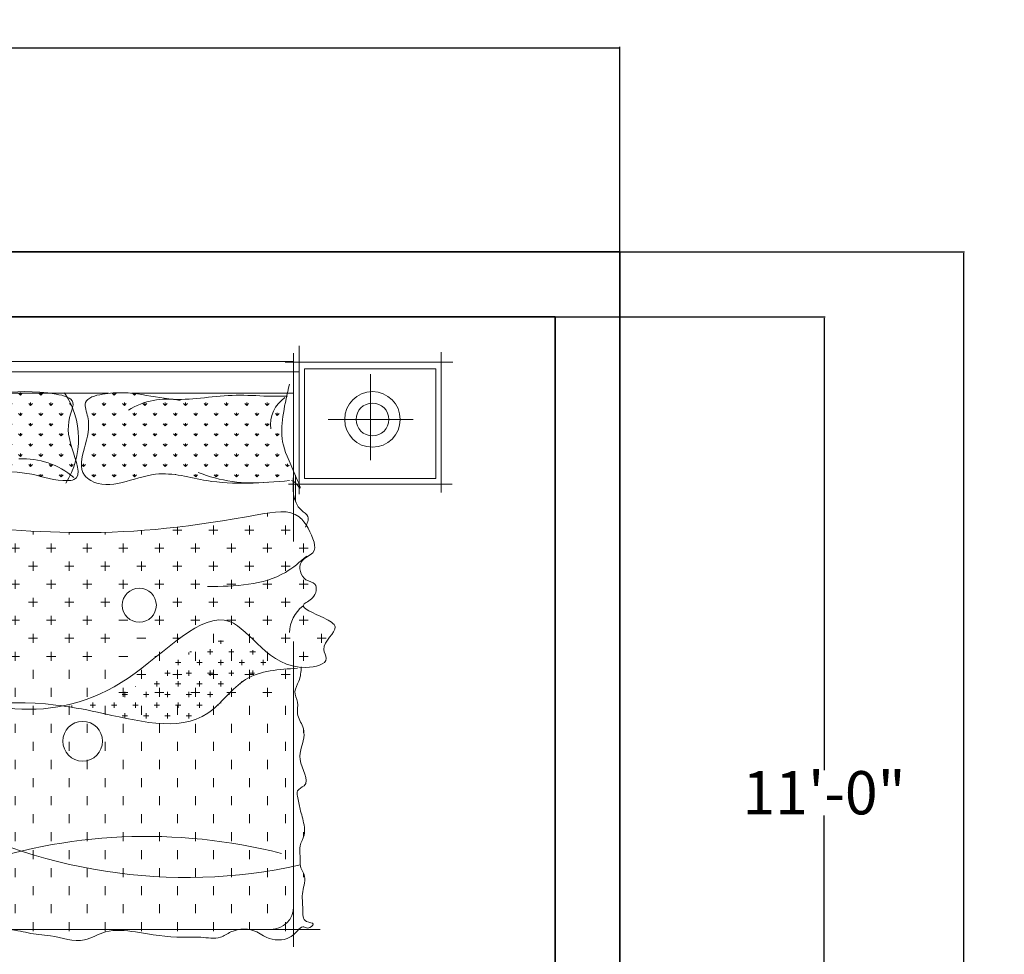
# Model space of a CAD drawing. Units: inches. Extents: x -26 to 575, y -18 to 513.
# Tile 28 of 28: x 439 to 575, y 378 to 508. Entities that reach past the tile are written whole.
import ezdxf

# ---------------------------------------------------------------- set-up
doc = ezdxf.new("R2010")
doc.units = ezdxf.units.IN
doc.header["$MEASUREMENT"] = 0
for name, color, linetype, lineweight in [('A-ANNO-DIMS', 2, 'Continuous', 18), ('A-WALL', 7, 'Continuous', 35), ('Furniture', 8, 'Continuous', 15)]:
    doc.layers.add(name, color=color, linetype=linetype, lineweight=lineweight)
doc.styles.get("Standard").update_dxf_attribs({"font": 'arial.ttf', "height": 6})
doc.dimstyles.get("Standard").update_dxf_attribs({"dimtxt": 6, "dimasz": 0.18, "dimexe": 0.18, "dimexo": 0.0625, "dimgap": 0.09, "dimtad": 0, "dimtih": 1, "dimtoh": 1, "dimzin": 0, "dimdsep": 46, "dimlunit": 3, "dimtxsty": 'Standard', "dimcen": 0.09, "dimadec": 0, "dimazin": 0, "dimtfac": 1, "dimtofl": 0, "dimtmove": 0, "dimatfit": 3, "dimfxl": 1, "dimtolj": 1, "dimtzin": 0, "dimarcsym": 0})

# ---------------------------------------------------------------- blocks, each defined once
blk = doc.blocks.new('*D1')
at = {"layer": 'A-ANNO-DIMS', "color": 0, "lineweight": -2, "transparency": 16777216}
for p, q in [((18.18, 475.57), (18.18, 503.94)), ((522.18, 475.57), (522.18, 503.94)), ((18.36, 503.76), (264.87, 503.76)), ((522, 503.76), (275.48, 503.76))]:
    blk.add_line(p, q, dxfattribs=at)
at = {"layer": 'A-ANNO-DIMS', "color": 0, "transparency": 16777216}
for points in [[(18.36, 503.79), (18.36, 503.73), (18.18, 503.76)], [(522, 503.79), (522, 503.73), (522.18, 503.76)]]:
    blk.add_solid(points, dxfattribs=at)
at = {"layer": 'Defpoints', "color": 0, "transparency": 16777216}
for p in [(522.18, 503.76), (18.18, 475.51), (522.18, 475.51)]:
    blk.add_point(p, dxfattribs=at)
at = {"layer": 'A-ANNO-DIMS', "color": 0, "transparency": 16777216, "insert": (270.18, 503.76), "char_height": 6, "attachment_point": 5}
blk.add_mtext("\\A1;42'", dxfattribs=at)
blk = doc.blocks.new('*D2')
at = {"layer": 'A-ANNO-DIMS', "color": 0, "lineweight": -2, "transparency": 16777216}
for p, q in [((522.24, 475.51), (569.98, 475.51)), ((569.8, 475.33), (569.8, 250.66)), ((569.8, 19.69), (569.8, 244.35)), ((522.24, 19.51), (569.98, 19.51))]:
    blk.add_line(p, q, dxfattribs=at)
at = {"layer": 'A-ANNO-DIMS', "color": 0, "transparency": 16777216}
for points in [[(569.77, 475.33), (569.83, 475.33), (569.8, 475.51)], [(569.77, 19.69), (569.83, 19.69), (569.8, 19.51)]]:
    blk.add_solid(points, dxfattribs=at)
at = {"layer": 'Defpoints', "color": 0, "transparency": 16777216}
for p in [(522.18, 475.51), (522.18, 19.51), (569.8, 19.51)]:
    blk.add_point(p, dxfattribs=at)
at = {"layer": 'A-ANNO-DIMS', "color": 0, "transparency": 16777216, "insert": (569.8, 247.51), "char_height": 6, "attachment_point": 5}
blk.add_mtext("\\A1;38'", dxfattribs=at)
blk = doc.blocks.new('BED-DOUBLE-WITH-NIGHTSTANDS')
for p, q in [((1.93, 83.36), (1.93, 62.76)), ((82.67, 83.36), (82.67, 62.76)), ((21.61, 63.03), (21.61, 82.46)), ((22.83, 60.83), (22.83, 82.62)), ((81.88, 82.34), (81.88, 56.23)), ((102.35, 63.03), (102.35, 82.46)), ((23.23, 81.08), (0, 81.08)), ((10.27, 81.76), (8.94, 70.83)), ((21.24, 81.17), (81.88, 81.17)), ((103.97, 81.08), (80.74, 81.08)), ((20.89, 80.15), (2.67, 80.15)), ((2.67, 80.15), (2.67, 64.97)), ((20.89, 64.97), (20.89, 80.15)), ((82.67, 79.72), (21.06, 79.72)), ((101.63, 80.15), (83.41, 80.15)), ((83.41, 80.15), (83.41, 64.97)), ((92.57, 79.4), (92.57, 67.51)), ((101.63, 64.97), (101.63, 80.15)), ((14.67, 76.01), (4.51, 77.26)), ((25.06, 76.76), (22.83, 76.76)), ((41.17, 76.51), (40.96, 76.72)), ((41.17, 76.51), (41.43, 76.77)), ((41.17, 76.51), (41.17, 76.74)), ((56.23, 76.76), (41.36, 76.76)), ((44, 76.51), (43.73, 76.77)), ((44, 76.51), (44, 76.88)), ((44, 76.51), (44.26, 76.77)), ((46.83, 76.51), (46.56, 76.77)), ((46.83, 76.51), (46.83, 76.88)), ((46.83, 76.51), (47.09, 76.77)), ((57, 76.51), (56.74, 76.77)), ((57, 76.51), (57, 76.83)), ((57, 76.51), (57.27, 76.77)), ((81.88, 76.76), (59.39, 76.76)), ((59.83, 76.51), (59.59, 76.74)), ((59.83, 76.51), (59.83, 76.72)), ((59.83, 76.51), (60.02, 76.69)), ((8.06, 67.24), (12.03, 75.72)), ((11.46, 75.32), (8.12, 68.2)), ((11.77, 75.18), (11.46, 75.32)), ((12.03, 75.72), (14.23, 74.69)), ((25.61, 75.09), (25.35, 75.36)), ((25.61, 75.09), (25.61, 75.47)), ((25.61, 75.09), (25.88, 75.36)), ((28.44, 75.09), (28.18, 75.36)), ((28.44, 75.09), (28.44, 75.47)), ((28.44, 75.09), (28.71, 75.36)), ((31.27, 75.09), (31, 75.36)), ((31.27, 75.09), (31.27, 75.47)), ((31.27, 75.09), (31.53, 75.36)), ((34.1, 75.09), (33.83, 75.36)), ((34.1, 75.09), (34.1, 75.47)), ((34.1, 75.09), (34.36, 75.36)), ((36.93, 75.09), (36.66, 75.36)), ((36.93, 75.09), (36.93, 75.47)), ((36.93, 75.09), (37.19, 75.36)), ((39.75, 75.09), (39.49, 75.36)), ((39.75, 75.09), (39.75, 75.47)), ((39.75, 75.09), (40.02, 75.36)), ((42.58, 75.09), (42.32, 75.36)), ((42.58, 75.09), (42.58, 75.47)), ((42.58, 75.09), (42.85, 75.36)), ((45.41, 75.09), (45.15, 75.36)), ((45.41, 75.09), (45.41, 75.47)), ((45.41, 75.09), (45.68, 75.36)), ((48.24, 75.09), (47.97, 75.36)), ((48.24, 75.09), (48.24, 75.47)), ((48.24, 75.09), (48.5, 75.36)), ((51.07, 75.09), (50.8, 75.36)), ((53, 75.34), (53.03, 75.36)), ((55.59, 75.09), (55.32, 75.36)), ((55.59, 75.09), (55.59, 75.47)), ((55.59, 75.09), (55.85, 75.36)), ((58.42, 75.09), (58.15, 75.36)), ((58.42, 75.09), (58.42, 75.47)), ((58.42, 75.09), (58.68, 75.36)), ((61.25, 75.09), (60.98, 75.36)), ((61.25, 75.09), (61.25, 75.47)), ((61.25, 75.09), (61.51, 75.36)), ((64.07, 75.09), (63.81, 75.36)), ((64.07, 75.09), (64.07, 75.47)), ((64.07, 75.09), (64.34, 75.36)), ((66.9, 75.09), (66.64, 75.36)), ((66.9, 75.09), (66.9, 75.47)), ((66.9, 75.09), (67.17, 75.36)), ((69.73, 75.09), (69.47, 75.36)), ((69.73, 75.09), (69.73, 75.47)), ((69.73, 75.09), (70, 75.36)), ((72.56, 75.09), (72.29, 75.36)), ((72.56, 75.09), (72.56, 75.47)), ((72.56, 75.09), (72.82, 75.36)), ((75.39, 75.09), (75.12, 75.36)), ((75.39, 75.09), (75.39, 75.47)), ((75.39, 75.09), (75.65, 75.36)), ((78.22, 75.09), (77.95, 75.36)), ((78.22, 75.09), (78.22, 75.47)), ((78.22, 75.09), (78.48, 75.36)), ((14.23, 74.69), (10.26, 66.21)), ((19.14, 71.73), (13.98, 74.14)), ((27.03, 73.68), (26.76, 73.94)), ((27.03, 73.68), (27.03, 74.05)), ((27.03, 73.68), (27.29, 73.94)), ((29.85, 73.68), (29.59, 73.94)), ((29.85, 73.68), (30.12, 73.94)), ((29.86, 73.68), (29.86, 74.05)), ((32.68, 73.68), (32.42, 73.94)), ((32.68, 73.68), (32.68, 74.05)), ((32.68, 73.68), (32.95, 73.94)), ((35.51, 73.68), (35.25, 73.94)), ((35.51, 73.68), (35.51, 74.05)), ((35.51, 73.68), (35.78, 73.94)), ((38.34, 73.68), (38.07, 73.94)), ((38.34, 73.68), (38.34, 74.05)), ((38.34, 73.68), (38.61, 73.94)), ((41.17, 73.68), (40.9, 73.94)), ((41.17, 73.68), (41.17, 74.05)), ((41.17, 73.68), (41.43, 73.94)), ((44, 73.68), (43.73, 73.94)), ((44, 73.68), (44, 74.05)), ((44, 73.68), (44.26, 73.94)), ((46.83, 73.68), (46.56, 73.94)), ((46.83, 73.68), (46.83, 74.05)), ((46.83, 73.68), (47.09, 73.94)), ((49.65, 73.68), (49.39, 73.94)), ((49.65, 73.68), (49.65, 74.05)), ((49.65, 73.68), (49.92, 73.94)), ((51.07, 75.09), (51.07, 75.1)), ((51.07, 75.09), (51.07, 75.1)), ((54.17, 73.68), (53.91, 73.94)), ((54.17, 73.68), (54.17, 74.05)), ((54.17, 73.68), (54.44, 73.94)), ((57, 73.68), (56.74, 73.94)), ((57, 73.68), (57, 74.05)), ((57, 73.68), (57.27, 73.94)), ((59.83, 73.68), (59.57, 73.94)), ((59.83, 73.68), (59.83, 74.05)), ((59.83, 73.68), (60.1, 73.94)), ((62.66, 73.68), (62.39, 73.94)), ((62.66, 73.68), (62.66, 74.05)), ((62.66, 73.68), (62.92, 73.94)), ((65.49, 73.68), (65.22, 73.94)), ((65.49, 73.68), (65.49, 74.05)), ((65.49, 73.68), (65.75, 73.94)), ((68.32, 73.68), (68.05, 73.94)), ((68.32, 73.68), (68.32, 74.05)), ((68.32, 73.68), (68.58, 73.94)), ((71.14, 73.68), (70.88, 73.94)), ((71.14, 73.68), (71.41, 73.94)), ((71.15, 73.68), (71.15, 74.05)), ((73.97, 73.68), (73.71, 73.94)), ((73.97, 73.68), (73.97, 74.05)), ((73.97, 73.68), (74.24, 73.94)), ((76.8, 73.68), (76.54, 73.94)), ((76.8, 73.68), (76.8, 74.05)), ((76.8, 73.68), (77.07, 73.94)), ((79.63, 73.68), (79.36, 73.94)), ((79.63, 73.68), (79.63, 74.05)), ((79.63, 73.68), (79.9, 73.94)), ((13.24, 72.57), (11.03, 73.6)), ((14.13, 73), (11.6, 67.59)), ((17.98, 71.2), (14.13, 73)), ((25.61, 72.26), (25.35, 72.53)), ((25.61, 72.26), (25.61, 72.64)), ((25.61, 72.26), (25.88, 72.53)), ((28.44, 72.26), (28.18, 72.53)), ((28.44, 72.26), (28.44, 72.64)), ((28.44, 72.26), (28.71, 72.53)), ((31.27, 72.26), (31, 72.53)), ((31.27, 72.26), (31.27, 72.64)), ((31.27, 72.26), (31.53, 72.53)), ((34.1, 72.26), (33.83, 72.53)), ((34.1, 72.26), (34.1, 72.64)), ((34.1, 72.26), (34.36, 72.53)), ((36.93, 72.26), (36.66, 72.53)), ((36.93, 72.26), (36.93, 72.64)), ((36.93, 72.26), (37.19, 72.53)), ((39.75, 72.26), (39.49, 72.53)), ((39.75, 72.26), (39.75, 72.64)), ((39.75, 72.26), (40.02, 72.53)), ((42.58, 72.26), (42.32, 72.53)), ((42.58, 72.26), (42.58, 72.64)), ((42.58, 72.26), (42.85, 72.53)), ((45.41, 72.26), (45.15, 72.53)), ((45.41, 72.26), (45.41, 72.64)), ((45.41, 72.26), (45.68, 72.53)), ((48.24, 72.26), (47.97, 72.53)), ((48.24, 72.26), (48.24, 72.64)), ((48.24, 72.26), (48.5, 72.53)), ((55.59, 72.26), (55.32, 72.53)), ((55.59, 72.26), (55.59, 72.64)), ((55.59, 72.26), (55.85, 72.53)), ((58.42, 72.26), (58.15, 72.53)), ((58.42, 72.26), (58.42, 72.64)), ((58.42, 72.26), (58.68, 72.53)), ((61.25, 72.26), (60.98, 72.53)), ((61.25, 72.26), (61.25, 72.64)), ((61.25, 72.26), (61.51, 72.53)), ((64.07, 72.26), (63.81, 72.53)), ((64.07, 72.26), (64.07, 72.64)), ((64.07, 72.26), (64.34, 72.53)), ((66.9, 72.26), (66.64, 72.53)), ((66.9, 72.26), (66.9, 72.64)), ((66.9, 72.26), (67.17, 72.53)), ((69.73, 72.26), (69.47, 72.53)), ((69.73, 72.26), (69.73, 72.64)), ((69.73, 72.26), (70, 72.53)), ((72.56, 72.26), (72.29, 72.53)), ((72.56, 72.26), (72.56, 72.64)), ((72.56, 72.26), (72.82, 72.53)), ((75.39, 72.26), (75.12, 72.53)), ((75.39, 72.26), (75.39, 72.64)), ((75.39, 72.26), (75.65, 72.53)), ((78.22, 72.26), (77.95, 72.53)), ((78.22, 72.26), (78.22, 72.64)), ((78.22, 72.26), (78.48, 72.53)), ((98.47, 73.14), (86.67, 73.14)), ((15.45, 65.79), (17.98, 71.2)), ((15.8, 64.6), (19.14, 71.73)), ((24.2, 70.85), (23.97, 71.08)), ((24.2, 70.85), (24.2, 71.23)), ((24.2, 70.85), (24.46, 71.12)), ((27.03, 70.85), (26.76, 71.12)), ((27.03, 70.85), (27.03, 71.23)), ((27.03, 70.85), (27.29, 71.12)), ((29.85, 70.85), (29.59, 71.12)), ((29.85, 70.85), (30.12, 71.12)), ((29.86, 70.85), (29.86, 71.23)), ((32.68, 70.85), (32.42, 71.12)), ((32.68, 70.85), (32.68, 71.23)), ((32.68, 70.85), (32.95, 71.12)), ((35.51, 70.85), (35.25, 71.12)), ((35.51, 70.85), (35.51, 71.23)), ((35.51, 70.85), (35.78, 71.12)), ((38.34, 70.85), (38.07, 71.12)), ((38.34, 70.85), (38.34, 71.23)), ((38.34, 70.85), (38.61, 71.12)), ((41.17, 70.85), (40.9, 71.12)), ((41.17, 70.85), (41.17, 71.23)), ((41.17, 70.85), (41.43, 71.12)), ((44, 70.85), (43.73, 71.12)), ((44, 70.85), (44, 71.23)), ((44, 70.85), (44.26, 71.12)), ((46.83, 70.85), (46.56, 71.12)), ((46.83, 70.85), (46.83, 71.23)), ((46.83, 70.85), (47.09, 71.12)), ((49.65, 70.85), (49.39, 71.12)), ((49.65, 70.85), (49.65, 71.23)), ((49.65, 70.85), (49.92, 71.12)), ((54.17, 70.85), (53.91, 71.12)), ((54.17, 70.85), (54.17, 71.23)), ((54.17, 70.85), (54.44, 71.12)), ((57, 70.85), (56.74, 71.12)), ((57, 70.85), (57, 71.23)), ((57, 70.85), (57.27, 71.12)), ((59.83, 70.85), (59.57, 71.12)), ((59.83, 70.85), (59.83, 71.23)), ((59.83, 70.85), (60.1, 71.12)), ((62.66, 70.85), (62.39, 71.12)), ((62.66, 70.85), (62.66, 71.23)), ((62.66, 70.85), (62.92, 71.12)), ((65.49, 70.85), (65.22, 71.12)), ((65.49, 70.85), (65.49, 71.23)), ((65.49, 70.85), (65.75, 71.12)), ((68.32, 70.85), (68.05, 71.12)), ((68.32, 70.85), (68.32, 71.23)), ((68.32, 70.85), (68.58, 71.12)), ((71.14, 70.85), (70.88, 71.12)), ((71.14, 70.85), (71.41, 71.12)), ((71.15, 70.85), (71.15, 71.23)), ((73.97, 70.85), (73.71, 71.12)), ((73.97, 70.85), (73.97, 71.23)), ((73.97, 70.85), (74.24, 71.12)), ((76.8, 70.85), (76.54, 71.12)), ((76.8, 70.85), (76.8, 71.23)), ((76.8, 70.85), (77.07, 71.12)), ((79.63, 70.85), (79.36, 71.12)), ((79.63, 70.85), (79.63, 71.23)), ((79.63, 70.85), (79.9, 71.12)), ((25.61, 69.44), (25.35, 69.7)), ((25.61, 69.44), (25.61, 69.81)), ((25.61, 69.44), (25.88, 69.7)), ((28.44, 69.44), (28.18, 69.7)), ((28.44, 69.44), (28.44, 69.81)), ((28.44, 69.44), (28.71, 69.7)), ((31.27, 69.44), (31, 69.7)), ((31.27, 69.44), (31.27, 69.81)), ((31.27, 69.44), (31.53, 69.7)), ((34.1, 69.44), (33.83, 69.7)), ((34.1, 69.44), (34.1, 69.81)), ((34.1, 69.44), (34.36, 69.7)), ((36.93, 69.44), (36.66, 69.7)), ((36.93, 69.44), (36.93, 69.81)), ((36.93, 69.44), (37.19, 69.7)), ((39.75, 69.44), (39.49, 69.7)), ((39.75, 69.44), (39.75, 69.81)), ((39.75, 69.44), (40.02, 69.7)), ((42.58, 69.44), (42.32, 69.7)), ((42.58, 69.44), (42.58, 69.81)), ((42.58, 69.44), (42.85, 69.7)), ((45.41, 69.44), (45.15, 69.7)), ((45.41, 69.44), (45.41, 69.81)), ((45.41, 69.44), (45.68, 69.7)), ((48.24, 69.44), (47.97, 69.7)), ((48.24, 69.44), (48.24, 69.81)), ((48.24, 69.44), (48.5, 69.7)), ((51.05, 69.45), (50.8, 69.7)), ((53.01, 69.68), (53.03, 69.7)), ((55.59, 69.44), (55.32, 69.7)), ((55.59, 69.44), (55.59, 69.81)), ((55.59, 69.44), (55.85, 69.7)), ((58.42, 69.44), (58.15, 69.7)), ((58.42, 69.44), (58.42, 69.81)), ((58.42, 69.44), (58.68, 69.7)), ((61.25, 69.44), (60.98, 69.7)), ((61.25, 69.44), (61.25, 69.81)), ((61.25, 69.44), (61.51, 69.7)), ((64.07, 69.44), (63.81, 69.7)), ((64.07, 69.44), (64.07, 69.81)), ((64.07, 69.44), (64.34, 69.7)), ((66.9, 69.44), (66.64, 69.7)), ((66.9, 69.44), (66.9, 69.81)), ((66.9, 69.44), (67.17, 69.7)), ((69.73, 69.44), (69.47, 69.7)), ((69.73, 69.44), (69.73, 69.81)), ((69.73, 69.44), (70, 69.7)), ((72.56, 69.44), (72.29, 69.7)), ((72.56, 69.44), (72.56, 69.81)), ((72.56, 69.44), (72.82, 69.7)), ((75.39, 69.44), (75.12, 69.7)), ((75.39, 69.44), (75.39, 69.81)), ((75.39, 69.44), (75.65, 69.7)), ((78.22, 69.44), (77.95, 69.7)), ((78.22, 69.44), (78.22, 69.81)), ((78.22, 69.44), (78.48, 69.7)), ((11.14, 68.07), (8.93, 69.1)), ((24.2, 68.02), (23.93, 68.29)), ((24.2, 68.02), (24.2, 68.4)), ((24.2, 68.02), (24.46, 68.29)), ((27.03, 68.02), (26.76, 68.29)), ((27.03, 68.02), (27.03, 68.4)), ((27.03, 68.02), (27.29, 68.29)), ((29.85, 68.02), (29.59, 68.29)), ((29.85, 68.02), (30.12, 68.29)), ((29.86, 68.02), (29.86, 68.4)), ((32.68, 68.02), (32.42, 68.29)), ((32.68, 68.02), (32.68, 68.4)), ((32.68, 68.02), (32.95, 68.29)), ((35.51, 68.02), (35.25, 68.29)), ((35.51, 68.02), (35.51, 68.4)), ((35.51, 68.02), (35.78, 68.29)), ((38.34, 68.02), (38.07, 68.29)), ((38.34, 68.02), (38.34, 68.4)), ((38.34, 68.02), (38.61, 68.29)), ((41.17, 68.02), (40.9, 68.29)), ((41.17, 68.02), (41.17, 68.4)), ((41.17, 68.02), (41.43, 68.29)), ((44, 68.02), (43.73, 68.29)), ((44, 68.02), (44, 68.4)), ((44, 68.02), (44.26, 68.29)), ((46.83, 68.02), (46.56, 68.29)), ((46.83, 68.02), (46.83, 68.4)), ((46.83, 68.02), (47.09, 68.29)), ((49.65, 68.02), (49.39, 68.29)), ((49.65, 68.02), (49.65, 68.4)), ((49.65, 68.02), (49.92, 68.29)), ((54.17, 68.02), (53.91, 68.29)), ((54.17, 68.02), (54.17, 68.4)), ((54.17, 68.02), (54.44, 68.29)), ((57, 68.02), (56.74, 68.29)), ((57, 68.02), (57, 68.4)), ((57, 68.02), (57.27, 68.29)), ((59.83, 68.02), (59.57, 68.29)), ((59.83, 68.02), (59.83, 68.4)), ((59.83, 68.02), (60.1, 68.29)), ((62.66, 68.02), (62.39, 68.29)), ((62.66, 68.02), (62.66, 68.4)), ((62.66, 68.02), (62.92, 68.29)), ((65.49, 68.02), (65.22, 68.29)), ((65.49, 68.02), (65.49, 68.4)), ((65.49, 68.02), (65.75, 68.29)), ((68.32, 68.02), (68.05, 68.29)), ((68.32, 68.02), (68.32, 68.4)), ((68.32, 68.02), (68.58, 68.29)), ((71.14, 68.02), (70.88, 68.29)), ((71.14, 68.02), (71.41, 68.29)), ((71.15, 68.02), (71.15, 68.4)), ((73.97, 68.02), (73.71, 68.29)), ((73.97, 68.02), (73.97, 68.4)), ((73.97, 68.02), (74.24, 68.29)), ((76.8, 68.02), (76.54, 68.29)), ((76.8, 68.02), (76.8, 68.4)), ((76.8, 68.02), (77.07, 68.29)), ((79.63, 68.02), (79.36, 68.29)), ((79.63, 68.02), (79.63, 68.4)), ((79.63, 68.02), (79.9, 68.29)), ((10.26, 66.21), (8.06, 67.24)), ((8.12, 68.2), (8.43, 68.05)), ((10.64, 67.02), (15.8, 64.6)), ((11.6, 67.59), (15.45, 65.79)), ((25.61, 66.61), (25.61, 66.98)), ((28.44, 66.61), (28.44, 66.98)), ((31.27, 66.61), (31.27, 66.98)), ((34.1, 66.61), (34.1, 66.98)), ((36.93, 66.61), (36.93, 66.98)), ((39.75, 66.61), (39.75, 66.98)), ((42.58, 66.61), (42.58, 66.98)), ((45.41, 66.61), (45.41, 66.98)), ((48.24, 66.61), (48.24, 66.98)), ((51.07, 66.61), (51.07, 66.98)), ((52.76, 66.61), (52.76, 66.98)), ((55.59, 66.61), (55.59, 66.98)), ((58.42, 66.61), (58.42, 66.98)), ((61.25, 66.61), (61.25, 66.98)), ((64.07, 66.61), (64.07, 66.98)), ((66.9, 66.61), (66.9, 66.98)), ((69.73, 66.61), (69.73, 66.98)), ((72.56, 66.61), (72.56, 66.98)), ((75.39, 66.61), (75.39, 66.98)), ((78.22, 66.61), (78.22, 66.98)), ((81.04, 66.61), (81.04, 66.98)), ((24.2, 65.39), (24.2, 65.57)), ((25.61, 66.61), (25.35, 66.87)), ((25.61, 66.61), (25.88, 66.87)), ((27.03, 65.19), (27.03, 65.57)), ((28.44, 66.61), (28.18, 66.87)), ((28.44, 66.61), (28.71, 66.87)), ((29.86, 65.19), (29.86, 65.57)), ((31.27, 66.61), (31, 66.87)), ((31.27, 66.61), (31.53, 66.87)), ((32.68, 65.19), (32.68, 65.57)), ((34.1, 66.61), (33.83, 66.87)), ((34.1, 66.61), (34.36, 66.87)), ((35.51, 65.39), (35.51, 65.57)), ((36.93, 66.61), (36.66, 66.87)), ((36.93, 66.61), (37.19, 66.87)), ((39.75, 66.61), (39.49, 66.87)), ((39.75, 66.61), (40.02, 66.87)), ((42.58, 66.61), (42.32, 66.87)), ((42.58, 66.61), (42.85, 66.87)), ((45.41, 66.61), (45.15, 66.87)), ((45.41, 66.61), (45.68, 66.87)), ((46.83, 65.23), (46.83, 65.57)), ((48.24, 66.61), (47.97, 66.87)), ((48.24, 66.61), (48.5, 66.87)), ((49.65, 65.19), (49.65, 65.57)), ((51.07, 66.61), (50.8, 66.87)), ((51.07, 66.61), (51.33, 66.87)), ((52.76, 66.61), (52.49, 66.87)), ((52.76, 66.61), (53.03, 66.87)), ((54.17, 65.19), (54.17, 65.57)), ((55.59, 66.61), (55.32, 66.87)), ((55.59, 66.61), (55.85, 66.87)), ((57, 65.19), (57, 65.57)), ((58.42, 66.61), (58.15, 66.87)), ((58.42, 66.61), (58.68, 66.87)), ((59.83, 65.19), (59.83, 65.57)), ((61.25, 66.61), (60.98, 66.87)), ((61.25, 66.61), (61.51, 66.87)), ((62.66, 65.52), (62.66, 65.57)), ((64.07, 66.61), (63.81, 66.87)), ((64.07, 66.61), (64.34, 66.87)), ((65.49, 65.48), (65.49, 65.57)), ((66.9, 66.61), (66.64, 66.87)), ((66.9, 66.61), (67.17, 66.87)), ((68.32, 65.19), (68.32, 65.57)), ((69.73, 66.61), (69.47, 66.87)), ((69.73, 66.61), (70, 66.87)), ((71.15, 65.19), (71.15, 65.57)), ((72.56, 66.61), (72.29, 66.87)), ((72.56, 66.61), (72.82, 66.87)), ((73.97, 65.19), (73.97, 65.57)), ((75.39, 66.61), (75.12, 66.87)), ((75.39, 66.61), (75.65, 66.87)), ((76.8, 65.19), (76.8, 65.57)), ((78.22, 66.61), (77.95, 66.87)), ((78.22, 66.61), (78.48, 66.87)), ((79.63, 65.19), (79.63, 65.57)), ((81.04, 66.61), (80.78, 66.87)), ((81.04, 66.61), (81.25, 66.82)), ((2.67, 64.97), (20.89, 64.97)), ((24.29, 65.29), (24.46, 65.46)), ((27.03, 65.19), (26.76, 65.46)), ((27.03, 65.19), (27.29, 65.46)), ((29.85, 65.19), (29.59, 65.46)), ((29.85, 65.19), (30.12, 65.46)), ((32.68, 65.19), (32.42, 65.46)), ((32.68, 65.19), (32.95, 65.46)), ((35.33, 65.37), (35.25, 65.46)), ((35.74, 65.42), (35.78, 65.46)), ((46.77, 65.25), (46.56, 65.46)), ((46.86, 65.22), (47.09, 65.46)), ((49.65, 65.19), (49.39, 65.46)), ((49.65, 65.19), (49.92, 65.46)), ((54.17, 65.19), (53.91, 65.46)), ((54.17, 65.19), (54.44, 65.46)), ((57, 65.19), (56.74, 65.46)), ((57, 65.19), (57.27, 65.46)), ((59.83, 65.19), (59.57, 65.46)), ((59.83, 65.19), (60.1, 65.46)), ((65.74, 65.45), (65.75, 65.46)), ((68.32, 65.19), (68.05, 65.46)), ((68.32, 65.19), (68.58, 65.46)), ((71.14, 65.19), (70.88, 65.46)), ((71.14, 65.19), (71.41, 65.46)), ((73.97, 65.19), (73.71, 65.46)), ((73.97, 65.19), (74.24, 65.46)), ((76.8, 65.19), (76.54, 65.46)), ((76.8, 65.19), (77.07, 65.46)), ((79.63, 65.19), (79.36, 65.46)), ((79.63, 65.19), (79.9, 65.46)), ((82.15, 61.74), (82.15, 65.42)), ((83.41, 64.97), (101.63, 64.97)), ((0.45, 64.15), (23.14, 64.15)), ((55.59, 64.12), (55.59, 64.15)), ((81.19, 64.15), (103.88, 64.15)), ((78.27, 59.67), (78.27, 60.15)), ((20.77, 58.21), (20.77, 58.42)), ((21.39, 57.79), (21.31, 57.79)), ((26.39, 57.79), (25.14, 57.79)), ((25.77, 57.17), (25.77, 58.42)), ((31.39, 57.79), (30.14, 57.79)), ((30.77, 57.17), (30.77, 58.42)), ((36.39, 57.79), (35.14, 57.79)), ((35.77, 57.17), (35.77, 58.41)), ((41.39, 57.79), (40.14, 57.79)), ((40.77, 57.17), (40.77, 57.97)), ((45.77, 57.17), (45.77, 57.64)), ((50.77, 57.17), (50.77, 57.46)), ((55.77, 57.17), (55.77, 57.48)), ((60.77, 57.17), (60.77, 57.74)), ((66.39, 57.79), (65.14, 57.79)), ((65.77, 57.17), (65.77, 58.21)), ((71.39, 57.79), (70.14, 57.79)), ((70.77, 57.17), (70.77, 58.42)), ((76.39, 57.79), (75.14, 57.79)), ((75.77, 57.17), (75.77, 58.42)), ((81.39, 57.79), (80.14, 57.79)), ((80.77, 57.17), (80.77, 58.42)), ((23.27, 54.64), (23.27, 55.76)), ((28.89, 55.29), (27.64, 55.29)), ((28.27, 54.67), (28.27, 55.92)), ((33.89, 55.29), (32.64, 55.29)), ((33.27, 54.67), (33.27, 55.92)), ((38.89, 55.29), (37.64, 55.29)), ((38.27, 54.67), (38.27, 55.92)), ((43.89, 55.29), (42.64, 55.29)), ((43.27, 54.67), (43.27, 55.92)), ((48.89, 55.29), (47.64, 55.29)), ((48.27, 54.67), (48.27, 55.92)), ((53.89, 55.29), (52.64, 55.29)), ((53.27, 54.67), (53.27, 55.92)), ((58.89, 55.29), (57.64, 55.29)), ((58.27, 54.67), (58.27, 55.92)), ((63.89, 55.29), (62.64, 55.29)), ((63.27, 54.67), (63.27, 55.92)), ((68.89, 55.29), (67.64, 55.29)), ((68.27, 54.67), (68.27, 55.92)), ((73.89, 55.29), (72.64, 55.29)), ((73.27, 54.67), (73.27, 55.92)), ((78.89, 55.29), (77.64, 55.29)), ((78.27, 54.67), (78.27, 55.92)), ((83.89, 55.29), (82.64, 55.29)), ((83.27, 54.67), (83.27, 55.92)), ((30.77, 52.17), (30.77, 53.42)), ((35.77, 52.17), (35.77, 53.42)), ((40.77, 52.17), (40.77, 53.42)), ((45.77, 52.17), (45.77, 53.42)), ((50.77, 52.17), (50.77, 53.42)), ((55.77, 52.17), (55.77, 53.42)), ((60.77, 52.17), (60.77, 53.42)), ((65.77, 52.17), (65.77, 53.42)), ((70.77, 52.17), (70.77, 53.42)), ((75.77, 52.17), (75.77, 53.42)), ((80.77, 52.17), (80.77, 53.42)), ((26.39, 52.79), (25.62, 52.79)), ((31.39, 52.79), (30.14, 52.79)), ((36.39, 52.79), (35.14, 52.79)), ((41.39, 52.79), (40.14, 52.79)), ((46.39, 52.79), (45.14, 52.79)), ((51.39, 52.79), (50.14, 52.79)), ((56.39, 52.79), (55.14, 52.79)), ((61.39, 52.79), (60.14, 52.79)), ((66.39, 52.79), (65.14, 52.79)), ((71.39, 52.79), (70.14, 52.79)), ((76.39, 52.79), (75.14, 52.79)), ((81.39, 52.79), (80.14, 52.79)), ((23.27, 49.67), (23.27, 50.92)), ((28.27, 49.67), (28.27, 50.92)), ((33.27, 49.67), (33.27, 50.92)), ((38.27, 49.67), (38.27, 50.92)), ((43.27, 49.67), (43.27, 50.92)), ((48.27, 49.67), (48.27, 50.92)), ((53.27, 49.67), (53.27, 50.92)), ((58.27, 49.67), (58.27, 50.92)), ((63.27, 49.67), (63.27, 50.92)), ((68.27, 49.67), (68.27, 50.92)), ((73.27, 49.67), (73.27, 50.92)), ((78.27, 49.67), (78.27, 50.92)), ((83.27, 49.67), (83.27, 50.92)), ((23.89, 50.29), (22.64, 50.29)), ((28.89, 50.29), (27.64, 50.29)), ((33.89, 50.29), (32.64, 50.29)), ((38.89, 50.29), (37.64, 50.29)), ((43.89, 50.29), (42.64, 50.29)), ((48.89, 50.29), (47.64, 50.29)), ((53.89, 50.29), (52.64, 50.29)), ((58.89, 50.29), (57.64, 50.29)), ((63.89, 50.29), (62.64, 50.29)), ((68.89, 50.29), (67.64, 50.29)), ((73.89, 50.29), (72.64, 50.29)), ((78.89, 50.29), (77.64, 50.29)), ((83.89, 50.29), (82.64, 50.29)), ((20.77, 47.17), (20.77, 48.42)), ((30.77, 47.17), (30.77, 48.42)), ((35.77, 47.17), (35.77, 48.42)), ((40.77, 47.17), (40.77, 48.42)), ((45.77, 47.17), (45.77, 48.42)), ((50.77, 47.17), (50.77, 48.42)), ((55.77, 47.17), (55.77, 48.42)), ((65.77, 47.17), (65.77, 48.42)), ((70.77, 47.17), (70.77, 48.42)), ((75.77, 47.17), (75.77, 48.42)), ((80.77, 47.17), (80.77, 48.42)), ((21.39, 47.79), (20.41, 47.79)), ((26.39, 47.79), (25.14, 47.79)), ((31.39, 47.79), (30.14, 47.79)), ((36.39, 47.79), (35.14, 47.79)), ((41.39, 47.79), (40.14, 47.79)), ((46.39, 47.79), (45.14, 47.79)), ((51.39, 47.79), (50.14, 47.79)), ((56.39, 47.79), (55.14, 47.79)), ((66.39, 47.79), (65.14, 47.79)), ((71.39, 47.79), (70.14, 47.79)), ((76.39, 47.79), (75.14, 47.79)), ((81.39, 47.79), (80.14, 47.79)), ((23.89, 45.29), (22.64, 45.29)), ((23.27, 44.67), (23.27, 45.92)), ((28.89, 45.29), (27.64, 45.29)), ((28.27, 44.67), (28.27, 45.92)), ((33.89, 45.29), (32.64, 45.29)), ((33.27, 44.67), (33.27, 45.92)), ((38.89, 45.29), (37.64, 45.29)), ((38.27, 44.67), (38.27, 45.92)), ((43.89, 45.29), (42.64, 45.29)), ((43.27, 44.67), (43.27, 45.92)), ((48.89, 45.29), (47.64, 45.29)), ((48.27, 44.67), (48.27, 45.92)), ((53.89, 45.29), (52.64, 45.29)), ((53.27, 44.67), (53.27, 45.92)), ((58.89, 45.29), (57.64, 45.29)), ((63.89, 45.29), (62.64, 45.29)), ((63.27, 44.67), (63.27, 45.92)), ((68.89, 45.29), (67.64, 45.29)), ((68.27, 44.67), (68.27, 45.92)), ((73.89, 45.29), (72.64, 45.29)), ((73.27, 44.67), (73.27, 45.92)), ((78.89, 45.29), (77.64, 45.29)), ((78.27, 44.67), (78.27, 45.92)), ((83.89, 45.29), (82.64, 45.29)), ((83.27, 44.67), (83.27, 45.92)), ((21.39, 42.79), (20.14, 42.79)), ((20.77, 42.17), (20.77, 43.42)), ((26.39, 42.79), (25.14, 42.79)), ((31.39, 42.79), (30.14, 42.79)), ((30.77, 42.17), (30.77, 43.42)), ((36.39, 42.79), (35.14, 42.79)), ((35.77, 42.17), (35.77, 43.42)), ((41.39, 42.79), (40.14, 42.79)), ((40.77, 42.17), (40.77, 43.42)), ((46.39, 42.79), (45.14, 42.79)), ((45.77, 42.17), (45.77, 43.42)), ((51.39, 42.79), (50.14, 42.79)), ((50.77, 42.17), (50.77, 43.42)), ((56.39, 42.79), (55.14, 42.79)), ((55.77, 42.17), (55.77, 43.42)), ((61.39, 42.79), (60.14, 42.79)), ((66.09, 42.79), (65.14, 42.79)), ((65.77, 42.17), (65.77, 43.42)), ((70.77, 42.17), (70.77, 43.42)), ((72.15, 42.39), (71.41, 42.39)), ((71.78, 42.02), (71.78, 42.49)), ((75.77, 42.17), (75.77, 43.42)), ((76.39, 42.79), (76.07, 42.79)), ((81.39, 42.79), (80.14, 42.79)), ((80.77, 42.17), (80.77, 43.42)), ((81.88, 42.36), (81.88, 0)), ((86.39, 42.79), (85.14, 42.79)), ((85.77, 42.17), (85.77, 43.42)), ((70.3, 40.54), (70.3, 41.28)), ((73.26, 40.54), (73.26, 41.28)), ((76.21, 40.54), (76.21, 41.13)), ((18.89, 40.29), (17.83, 40.29)), ((18.27, 39.67), (18.27, 40.92)), ((23.89, 40.29), (22.64, 40.29)), ((23.27, 39.99), (23.27, 40.92)), ((28.89, 40.29), (27.64, 40.29)), ((28.27, 39.67), (28.27, 40.92)), ((33.89, 40.29), (32.64, 40.29)), ((33.27, 39.67), (33.27, 40.92)), ((38.89, 40.29), (37.64, 40.29)), ((38.27, 39.67), (38.27, 40.92)), ((43.89, 40.29), (42.64, 40.29)), ((43.27, 39.67), (43.27, 40.92)), ((48.89, 40.29), (47.64, 40.29)), ((48.27, 39.67), (48.27, 40.92)), ((53.89, 40.29), (52.64, 40.29)), ((53.27, 39.67), (53.27, 40.92)), ((58.89, 40.29), (57.64, 40.29)), ((62.9, 40.29), (62.64, 40.29)), ((63.27, 39.67), (63.27, 40.92)), ((65.87, 39.06), (65.87, 39.8)), ((67.35, 40.54), (67.35, 40.84)), ((67.72, 40.91), (67.48, 40.91)), ((68.27, 39.67), (68.27, 40.92)), ((68.83, 39.06), (68.83, 39.8)), ((70.67, 40.91), (69.93, 40.91)), ((71.78, 39.06), (71.78, 39.8)), ((73.62, 40.91), (72.89, 40.91)), ((73.27, 39.67), (73.27, 40.92)), ((74.73, 39.06), (74.73, 39.8)), ((76.58, 40.91), (75.84, 40.91)), ((77.68, 39.06), (77.68, 39.8)), ((78.27, 39.67), (78.27, 40.92)), ((83.89, 40.29), (82.64, 40.29)), ((83.27, 39.67), (83.27, 40.92)), ((22.83, 3.42), (22.83, 38.86)), ((25.77, 37.17), (25.77, 38.42)), ((30.77, 37.17), (30.77, 38.42)), ((35.77, 37.17), (35.77, 38.42)), ((40.77, 37.17), (40.77, 38.42)), ((45.77, 37.17), (45.77, 38.42)), ((50.77, 37.17), (50.77, 38.42)), ((55.77, 37.17), (55.77, 38.42)), ((60.77, 37.17), (60.77, 38.42)), ((64.4, 37.59), (64.4, 38.33)), ((66.24, 39.43), (65.5, 39.43)), ((65.77, 37.17), (65.77, 38.42)), ((67.35, 37.59), (67.35, 38.33)), ((69.2, 39.43), (68.46, 39.43)), ((70.3, 37.59), (70.3, 38.33)), ((70.77, 37.17), (70.77, 38.42)), ((72.15, 39.43), (71.41, 39.43)), ((73.26, 37.59), (73.26, 38.33)), ((75.1, 39.43), (74.36, 39.43)), ((75.77, 37.17), (75.77, 38.42)), ((76.21, 37.8), (76.21, 38.33)), ((78.05, 39.43), (77.32, 39.43)), ((80.77, 37.17), (80.77, 38.42)), ((61.39, 37.79), (60.14, 37.79)), ((64.77, 37.96), (64.03, 37.96)), ((66.39, 37.79), (65.14, 37.79)), ((67.72, 37.96), (66.98, 37.96)), ((70.67, 37.96), (69.93, 37.96)), ((71.39, 37.79), (70.14, 37.79)), ((73.62, 37.96), (72.89, 37.96)), ((76.39, 37.79), (75.14, 37.79)), ((76.45, 37.96), (75.84, 37.96)), ((81.39, 37.79), (80.14, 37.79)), ((28.27, 34.67), (28.27, 35.92)), ((33.27, 34.67), (33.27, 35.92)), ((38.27, 34.67), (38.27, 35.92)), ((43.27, 34.67), (43.27, 35.92)), ((48.27, 34.67), (48.27, 35.92)), ((53.27, 34.67), (53.27, 35.92)), ((58.27, 34.67), (58.27, 35.92)), ((59.97, 36.11), (59.97, 36.16)), ((63.29, 36.48), (62.55, 36.48)), ((62.92, 36.11), (62.92, 36.85)), ((63.27, 34.67), (63.27, 35.92)), ((66.24, 36.48), (65.5, 36.48)), ((65.87, 36.11), (65.87, 36.85)), ((68.27, 34.67), (68.27, 35.92)), ((69.2, 36.48), (68.46, 36.48)), ((68.83, 36.11), (68.83, 36.85)), ((72.15, 36.48), (71.41, 36.48)), ((71.78, 36.11), (71.78, 36.85)), ((73.27, 34.67), (73.27, 35.92)), ((74.53, 36.48), (74.36, 36.48)), ((74.73, 36.66), (74.73, 36.85)), ((78.27, 34.67), (78.27, 35.92)), ((17.66, 35.29), (17.64, 35.29)), ((58.89, 35.29), (57.64, 35.29)), ((58.86, 35), (58.12, 35)), ((58.49, 34.64), (58.49, 35.37)), ((61.81, 35), (61.08, 35)), ((61.44, 34.64), (61.44, 35.37)), ((63.89, 35.29), (62.64, 35.29)), ((64.77, 35), (64.03, 35)), ((64.4, 34.64), (64.4, 35.37)), ((67.72, 35), (66.98, 35)), ((67.35, 34.64), (67.35, 35.37)), ((68.89, 35.29), (67.64, 35.29)), ((70.67, 35), (69.93, 35)), ((70.3, 34.64), (70.3, 35.37)), ((73.89, 35.29), (72.64, 35.29)), ((73.01, 35), (72.89, 35)), ((73.26, 35.25), (73.26, 35.37)), ((78.89, 35.29), (77.64, 35.29)), ((25.77, 32.17), (25.77, 33.42)), ((30.77, 32.17), (30.77, 33.42)), ((35.77, 32.17), (35.77, 33.42)), ((40.77, 32.17), (40.77, 33.42)), ((45.77, 32.17), (45.77, 33.42)), ((50.77, 32.17), (50.77, 33.42)), ((51.11, 33.25), (51.11, 33.48)), ((54.43, 33.53), (53.69, 33.53)), ((54.06, 33.16), (54.06, 33.9)), ((55.77, 32.17), (55.77, 33.42)), ((57.38, 33.53), (56.65, 33.53)), ((57.02, 33.16), (57.02, 33.9)), ((60.34, 33.53), (59.6, 33.53)), ((59.97, 33.16), (59.97, 33.9)), ((60.77, 32.17), (60.77, 33.42)), ((63.29, 33.53), (62.55, 33.53)), ((62.92, 33.16), (62.92, 33.9)), ((66.24, 33.53), (65.5, 33.53)), ((65.77, 32.17), (65.77, 33.42)), ((65.87, 33.16), (65.87, 33.9)), ((69.2, 33.53), (68.46, 33.53)), ((68.83, 33.16), (68.83, 33.9)), ((70.77, 32.17), (70.77, 33.42)), ((71.47, 33.53), (71.41, 33.53)), ((71.78, 33.81), (71.78, 33.9)), ((75.77, 32.17), (75.77, 33.42)), ((80.77, 32.17), (80.77, 33.42)), ((55.54, 32.37), (55.54, 32.42)), ((58.86, 32.05), (58.12, 32.05)), ((58.49, 31.74), (58.49, 32.42)), ((61.81, 32.05), (61.08, 32.05)), ((61.44, 31.68), (61.44, 32.42)), ((64.77, 32.05), (64.03, 32.05)), ((64.4, 31.68), (64.4, 32.42)), ((67.72, 32.05), (66.98, 32.05)), ((67.35, 31.68), (67.35, 32.42)), ((28.27, 29.67), (28.27, 30.92)), ((33.27, 29.67), (33.27, 30.92)), ((38.27, 29.67), (38.27, 30.92)), ((43.27, 29.67), (43.27, 30.92)), ((48.27, 29.67), (48.27, 30.92)), ((53.27, 29.67), (53.27, 30.92)), ((58.27, 29.67), (58.27, 30.92)), ((63.27, 29.67), (63.27, 30.92)), ((68.27, 29.67), (68.27, 30.92)), ((73.27, 29.67), (73.27, 30.92)), ((78.27, 29.67), (78.27, 30.92)), ((83.27, 29.67), (83.27, 30.11)), ((25.77, 27.17), (25.77, 28.42)), ((30.77, 27.17), (30.77, 28.42)), ((35.77, 27.17), (35.77, 28.42)), ((40.77, 27.17), (40.77, 28.42)), ((45.77, 27.17), (45.77, 28.42)), ((50.77, 27.17), (50.77, 28.42)), ((55.77, 27.17), (55.77, 28.42)), ((60.77, 27.17), (60.77, 28.42)), ((65.77, 27.17), (65.77, 28.42)), ((70.77, 27.17), (70.77, 28.42)), ((75.77, 27.17), (75.77, 28.42)), ((80.77, 27.17), (80.77, 28.42)), ((28.27, 24.67), (28.27, 25.92)), ((33.27, 24.67), (33.27, 25.92)), ((38.27, 24.67), (38.27, 25.92)), ((43.27, 24.67), (43.27, 25.92)), ((48.27, 24.67), (48.27, 25.92)), ((53.27, 24.67), (53.27, 25.92)), ((58.27, 24.67), (58.27, 25.92)), ((63.27, 24.67), (63.27, 25.92)), ((68.27, 24.67), (68.27, 25.92)), ((73.27, 24.67), (73.27, 25.92)), ((78.27, 24.67), (78.27, 25.92)), ((25.77, 22.17), (25.77, 23.42)), ((30.77, 22.17), (30.77, 23.42)), ((35.77, 22.17), (35.77, 23.42)), ((40.77, 22.17), (40.77, 23.42)), ((45.77, 22.17), (45.77, 23.42)), ((50.77, 22.17), (50.77, 23.42)), ((55.77, 22.17), (55.77, 23.42)), ((60.77, 22.17), (60.77, 23.42)), ((65.77, 22.17), (65.77, 23.42)), ((70.77, 22.17), (70.77, 23.42)), ((75.77, 22.17), (75.77, 23.42)), ((80.77, 22.17), (80.77, 23.42)), ((28.27, 19.67), (28.27, 20.92)), ((33.27, 19.67), (33.27, 20.92)), ((38.27, 19.67), (38.27, 20.92)), ((43.27, 19.67), (43.27, 20.92)), ((48.27, 19.67), (48.27, 20.92)), ((53.27, 19.67), (53.27, 20.92)), ((58.27, 19.67), (58.27, 20.92)), ((63.27, 19.67), (63.27, 20.92)), ((68.27, 19.67), (68.27, 20.92)), ((73.27, 19.67), (73.27, 20.92)), ((78.27, 19.67), (78.27, 20.92)), ((25.77, 17.17), (25.77, 18.42)), ((30.77, 17.17), (30.77, 18.42)), ((35.77, 17.17), (35.77, 18.42)), ((40.77, 17.17), (40.77, 18.42)), ((45.77, 17.17), (45.77, 18.42)), ((50.77, 17.17), (50.77, 18.42)), ((55.77, 17.17), (55.77, 18.42)), ((60.77, 17.17), (60.77, 18.42)), ((65.77, 17.17), (65.77, 18.42)), ((70.77, 17.17), (70.77, 18.42)), ((75.77, 17.17), (75.77, 18.42)), ((80.77, 17.17), (80.77, 18.42)), ((28.27, 14.67), (28.27, 15.92)), ((33.27, 14.67), (33.27, 15.92)), ((38.27, 14.67), (38.27, 15.92)), ((43.27, 14.67), (43.27, 15.92)), ((48.27, 14.67), (48.27, 15.92)), ((53.27, 14.67), (53.27, 15.92)), ((58.27, 14.67), (58.27, 15.92)), ((63.27, 14.67), (63.27, 15.92)), ((68.27, 14.67), (68.27, 15.92)), ((73.27, 14.67), (73.27, 15.92)), ((78.27, 14.67), (78.27, 15.92)), ((83.27, 15.26), (83.27, 15.92)), ((25.77, 12.17), (25.77, 13.42)), ((30.77, 12.17), (30.77, 13.42)), ((35.77, 12.17), (35.77, 13.42)), ((40.77, 12.17), (40.77, 13.42)), ((45.77, 12.17), (45.77, 13.42)), ((50.77, 12.17), (50.77, 13.42)), ((55.77, 12.17), (55.77, 13.42)), ((60.77, 12.17), (60.77, 13.42)), ((65.77, 12.17), (65.77, 13.42)), ((70.77, 12.17), (70.77, 13.42)), ((75.77, 12.17), (75.77, 13.42)), ((80.77, 12.17), (80.77, 13.42)), ((28.27, 9.67), (28.27, 10.92)), ((33.27, 9.67), (33.27, 10.92)), ((38.27, 9.67), (38.27, 10.92)), ((43.27, 9.67), (43.27, 10.92)), ((48.27, 9.67), (48.27, 10.92)), ((53.27, 9.67), (53.27, 10.92)), ((58.27, 9.67), (58.27, 10.92)), ((63.27, 9.67), (63.27, 10.92)), ((68.27, 9.67), (68.27, 10.92)), ((73.27, 9.67), (73.27, 10.92)), ((78.27, 9.67), (78.27, 10.92)), ((83.27, 9.67), (83.27, 10.2)), ((25.77, 7.17), (25.77, 8.42)), ((30.77, 7.17), (30.77, 8.42)), ((35.77, 7.17), (35.77, 8.42)), ((40.77, 7.17), (40.77, 8.42)), ((45.77, 7.17), (45.77, 8.42)), ((50.77, 7.17), (50.77, 8.42)), ((55.77, 7.17), (55.77, 8.42)), ((60.77, 7.17), (60.77, 8.42)), ((65.77, 7.17), (65.77, 8.42)), ((70.77, 7.17), (70.77, 8.42)), ((75.77, 7.17), (75.77, 8.42)), ((80.77, 7.17), (80.77, 8.42)), ((22.12, 7.87), (21.71, 7.87)), ((28.27, 4.67), (28.27, 5.92)), ((33.27, 4.67), (33.27, 5.92)), ((38.27, 4.67), (38.27, 5.92)), ((43.27, 4.67), (43.27, 5.92)), ((48.27, 4.67), (48.27, 5.92)), ((53.27, 4.67), (53.27, 5.92)), ((58.27, 4.67), (58.27, 5.92)), ((63.27, 4.67), (63.27, 5.92)), ((68.27, 4.67), (68.27, 5.92)), ((73.27, 4.67), (73.27, 5.92)), ((78.27, 4.67), (78.27, 5.92)), ((25.77, 2.17), (25.77, 3.42)), ((30.77, 2.46), (30.77, 3.42)), ((36.39, 2.79), (35.14, 2.79)), ((35.77, 3), (35.77, 3.42)), ((40.4, 2.79), (40.14, 2.79)), ((40.77, 2.75), (40.77, 3.42)), ((45.77, 2.17), (45.77, 3.42)), ((50.77, 2.17), (50.77, 3.42)), ((55.77, 2.17), (55.77, 3.42)), ((60.77, 2.17), (60.77, 3.42)), ((65.77, 2.17), (65.77, 3.42)), ((70.77, 2.17), (70.77, 3.42)), ((75.77, 2.41), (75.77, 3.42)), ((80.77, 2.17), (80.77, 3.42)), ((85.58, 2.43), (23.7, 2.43))]:
    blk.add_line(p, q)
for centre, radius in [((9.65, 76.68), 4.06), ((9.65, 76.68), 3.73), ((9.65, 76.68), 1.87), ((9.65, 76.68), 1.7), ((92.82, 73.14), 3.85), ((92.82, 73.14), 2.27), ((60.49, 47.37), 2.36), ((52.63, 28.52), 2.75)]:
    blk.add_circle(centre, radius)
for centre, radius, start, end in [((40.61, 70.41), 11.46, 327.7555, 34.1397), ((18.64, 72.67), 7.53, 354.3248, 27.7728), ((41.09, 50.38), 26, 95.0264, 117.3299), ((64.24, 66.16), 9.79, 78.7884, 122.5362), ((83.34, 72.35), 4.66, 124.7345, 186.5526), ((44.42, 57.1), 10.59, 48.8713, 93.3448), ((76.2, 84.7), 20.36, 248.1857, 275.9106), ((27.06, 44.47), 7.56, 311.0401, 36.1384), ((86.26, 43.42), 4.94, 128.8354, 178.0038), ((39.78, 19.64), 17.21, 170.0678, 270.9321), ((30.83, 21.41), 8.01, 183.5361, 317.8486), ((66.97, 82.6), 72.97, 239.8126, 282.5472), ((41.05, 10.13), 8.24, 134.2353, 249.0585), ((61.48, -60.53), 75.85, 75.7143, 109.4459), ((25.97, 5.58), 3.15, 180, 270), ((78.73, 5.58), 3.15, 270, 0)]:
    blk.add_arc(centre, radius, start, end)
for points, knots in [([(81.3, 78.04), (80.68, 75.31), (79.67, 70.85), (81.18, 67.62), (83.38, 62.52), (82.09, 64.57), (81.59, 64.66)], [0, 0, 0, 0, 7.603099, 12.404488, 14.892294, 16.432626, 16.432626, 16.432626, 16.432626]), ([(25.07, 76.86), (24.73, 74.84), (24.15, 71.41), (22.76, 66.41), (24.85, 64.9), (25.6, 63.75), (26.07, 63.83)], [0, 0, 0, 0, 6.47304, 11.006869, 12.799679, 14.2185, 14.2185, 14.2185, 14.2185]), ([(24.71, 64.66), (26.06, 64.63), (33, 64.48), (41.95, 67.2), (49.02, 64.48), (52.79, 64.86), (50.63, 69.88), (50.43, 72.76), (51.76, 76.03), (43.45, 78.05), (36.59, 75.07), (28.31, 76.39), (25.37, 76.36), (24.84, 76.35)], [0, 0, 0, 0, 4.049674, 20.880819, 25.932041, 26.821979, 31.217024, 36.043065, 37.533831, 40.150607, 55.448466, 62.672935, 64.278467, 64.278467, 64.278467, 64.278467]), ([(81.33, 64.66), (77.47, 64.34), (71.21, 63.83), (62.27, 66.78), (55.98, 62.89), (52.05, 65.92), (52.93, 69.57), (53.86, 72.57), (52.44, 75.93), (58.7, 77.69), (63.65, 75.45), (70.13, 76.24), (74.45, 76.62), (78.12, 76.32), (80.32, 76.35), (81.04, 76.35)], [0, 0, 0, 0, 11.502554, 18.635017, 27.654655, 28.800011, 32.595859, 36.914018, 38.927328, 41.544104, 52.009639, 56.262652, 60.661637, 65.075538, 67.252844, 67.252844, 67.252844, 67.252844]), ([(81.88, 65.42), (81.77, 63.58), (81.62, 61.27), (84.25, 59.71), (83.77, 58.74), (83.52, 58.22)], [0, 0, 0, 0, 4.973031, 6.254082, 7.747585, 7.747585, 7.747585, 7.747585]), ([(83.91, 58.07), (84.56, 56.74), (85.58, 54.64), (82.28, 53.65), (82.99, 50.72), (85.33, 50.53), (84.9, 48.23), (82.06, 47.25), (85.77, 45.87), (88.76, 44.17), (85.37, 42.03), (87.05, 39.3), (78.86, 37.34), (72.98, 51.01), (54.08, 29.24), (35.91, 32.92), (20.82, 41.99), (17.17, 32.57), (16.24, 37.8), (18.71, 38.79), (15.91, 43.44), (22.37, 43.45), (20.93, 46.18), (20.19, 47.95), (20.32, 52.93), (35.13, 52.6), (16.25, 58.94), (26.31, 59.48), (35.16, 58.38), (54.32, 56.67), (69.44, 58.46), (82.07, 60.88), (83.53, 58.65), (83.91, 58.07)], [0, 0, 0, 0, 3.481099, 5.475811, 8.043407, 9.436812, 11.330727, 12.888379, 16.258255, 18.252967, 21.734596, 23.018392, 26.087149, 38.445812, 54.5649, 86.600283, 92.594507, 98.286547, 100.905288, 101.70342, 105.471876, 109.954916, 110.954151, 113.598333, 116.114301, 124.231953, 133.25029, 137.509046, 143.991555, 164.906349, 189.961005, 195.579007, 197.573325, 197.573325, 197.573325, 197.573325]), ([(23.43, 55.19), (24.49, 55), (27.11, 54.54), (29.42, 53.18), (30.79, 52.36)], [0, 0, 0, 0, 3.194191, 7.94245, 7.94245, 7.94245, 7.94245]), ([(83.72, 54.2), (82.76, 53.38), (78.97, 50.14), (73.79, 50.03), (69.93, 49.96)], [0, 0, 0, 0, 3.737027, 14.742384, 14.742384, 14.742384, 14.742384]), ([(82.45, 38.63), (79.86, 38.49), (74.81, 38.21), (68.7, 28.86), (57.63, 32.1), (43.09, 34.7), (32.13, 32.98), (18.89, 30.82), (17.48, 34.15), (16.98, 35.35)], [0, 0, 0, 0, 7.385187, 14.402621, 29.694422, 35.583277, 59.348121, 65.733553, 69.320983, 69.320983, 69.320983, 69.320983]), ([(82.95, 38.85), (82.91, 38.17), (82.85, 36.97), (81.76, 35.43), (82.66, 33.92), (82.17, 32.16), (83.17, 30.81), (83.54, 28.6), (81.84, 26.13), (84.59, 22.62), (82.27, 21.86), (82.5, 20.48), (82.77, 18.98), (83.36, 17.21), (83.5, 15.41), (82.61, 14.09), (82.87, 12.46), (82.71, 11.04), (83.72, 9.61), (82.91, 7.55), (83.23, 5.58), (83.08, 3.39), (85.08, 3.34), (83.88, 2.36), (83.09, 3.04), (82.19, 1.93), (80.71, 0.69), (78.27, 1.05), (76.16, 2.63), (73.68, 2.58), (71.48, 0.95), (69.05, 1.47), (65.15, 1.19), (60.81, 2), (56.05, 2.59), (52.45, 0.27), (49.19, 1.51), (46.12, 1.7), (37.69, 3.67), (31.84, 3.18), (20.44, -0.09), (22.21, 3.75), (19.18, -0.44), (22.91, 0.39), (27.14, 0.63), (21.63, 1.85), (19.68, 4.27), (19.87, 11.16), (24.26, 3.84), (20.3, 10.76), (23.26, 12.85), (24.33, 17.43), (16.78, 17.59), (25.96, 19.23), (16.2, 20.68), (24.67, 22.01), (20.04, 24.96), (24.6, 28.15), (20.03, 29.6), (23.48, 31.6), (22.43, 34.55), (22.92, 41.18), (22.85, 37.06), (22.83, 35.35)], [0, 0, 0, 0, 2.033881, 3.581387, 5.07489, 6.704853, 8.655612, 9.757262, 13.24098, 16.903694, 18.063816, 18.788243, 20.635227, 22.875483, 24.324336, 25.871843, 27.320698, 29.140811, 29.950855, 32.312207, 34.847704, 36.565952, 37.541804, 38.447727, 39.194923, 40.100844, 41.912688, 45.194843, 46.251388, 49.875946, 51.496686, 54.215105, 56.7523, 63.316606, 67.484853, 70.581422, 75.324573, 76.965649, 79.915763, 100.671038, 102.483321, 104.317501, 106.523635, 109.038061, 111.571263, 115.809372, 117.667229, 122.411431, 125.445794, 129.976907, 132.758854, 136.424739, 139.918708, 143.481583, 147.135325, 151.002466, 153.252794, 157.23352, 159.244583, 161.905351, 164.097269, 169.015093, 172.531686, 172.531686, 172.531686, 172.531686])]:
    blk.add_open_spline(points, degree=3, knots=knots)
blk = doc.blocks.new('*D49')
at = {"layer": 'A-ANNO-DIMS', "color": 0, "lineweight": -2, "transparency": 16777216}
for p, q in [((278.24, 466.51), (550.66, 466.51)), ((550.48, 466.33), (550.48, 403.66)), ((550.48, 334.69), (550.48, 397.35)), ((278.24, 334.51), (550.66, 334.51))]:
    blk.add_line(p, q, dxfattribs=at)
at = {"layer": 'A-ANNO-DIMS', "color": 0, "transparency": 16777216}
for points in [[(550.45, 466.33), (550.51, 466.33), (550.48, 466.51)], [(550.45, 334.69), (550.51, 334.69), (550.48, 334.51)]]:
    blk.add_solid(points, dxfattribs=at)
at = {"layer": 'Defpoints', "color": 0, "transparency": 16777216}
for p in [(278.18, 466.51), (550.48, 466.51), (278.18, 334.51)]:
    blk.add_point(p, dxfattribs=at)
at = {"layer": 'A-ANNO-DIMS', "color": 0, "transparency": 16777216, "insert": (550.48, 400.51), "char_height": 6, "attachment_point": 5}
blk.add_mtext('\\A1;11\'-0"', dxfattribs=at)

msp = doc.modelspace()

# ---------------------------------------------------------------- linework, layer by layer
at = {"layer": 'A-WALL'}
for p, q in [((513.177, 466.508), (378.677, 466.508)), ((513.177, 334.508), (513.177, 466.508))]:
    msp.add_line(p, q, dxfattribs=at)
msp.add_lwpolyline([(18.177, 19.508), (522.177, 19.508), (522.177, 475.508), (18.177, 475.508)], close=True, dxfattribs=at)

# ---------------------------------------------------------------- block references
at = {"layer": 'Furniture'}
msp.add_blockref('BED-DOUBLE-WITH-NIGHTSTANDS', (395.028, 379.13), dxfattribs=at)

# ---------------------------------------------------------------- dimensions: what is measured, and where the dimension line sits
at = {"layer": 'A-ANNO-DIMS'}
dim = msp.add_linear_dim(base=(522.177, 503.757), p1=(18.177, 475.508), p2=(522.177, 475.508), dimstyle='Standard', override={"dimclrd": 0, "dimclre": 0, "dimclrt": 0}, dxfattribs=at)
dim.commit()
dim.dimension.update_dxf_attribs({"geometry": '*D1', "text_midpoint": (270.177, 503.757)})
for base, p1, p2, override, picture, middle in [((569.801, 19.508), (522.177, 475.508), (522.177, 19.508), {"dimclrd": 0, "dimclre": 0, "dimclrt": 0}, '*D2', (569.801, 247.508)), ((550.477, 466.508), (278.177, 334.508), (278.177, 466.508), {"dimdec": 1, "dimlfac": 1, "dimrnd": 0, "dimzin": 1, "dimdsep": 46, "dimlunit": 4, "dimfrac": 2}, '*D49', (550.477, 400.508))]:
    dim = msp.add_linear_dim(base=base, p1=p1, p2=p2, angle=90, dimstyle='Standard', override=override, dxfattribs=at)
    dim.commit()
    dim.dimension.update_dxf_attribs({"geometry": picture, "text_midpoint": middle})

doc.saveas('drawing.dxf')
